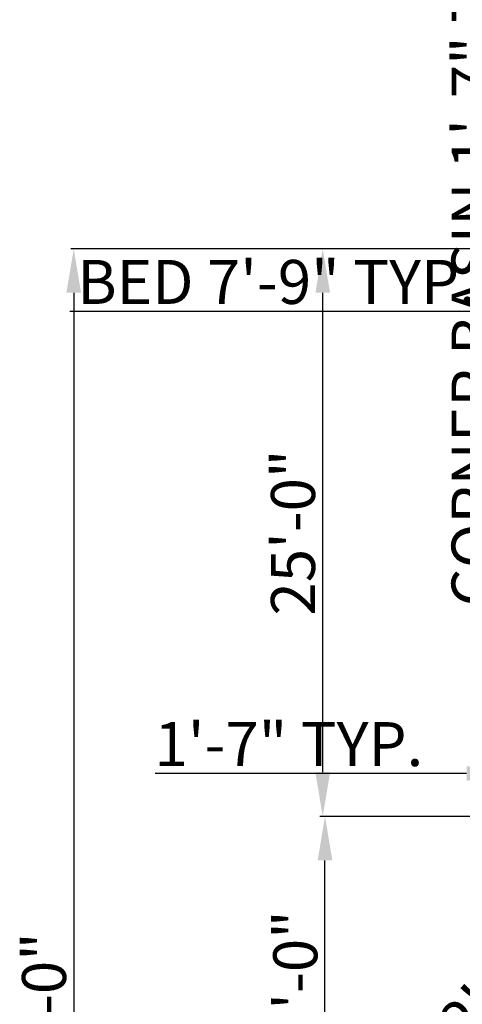
# Model space of a CAD drawing. Units: inches. Extents: x 2043 to 3177, y 1429 to 2563.
# Tile 9 of 14: x 2043 to 2224, y 1952 to 2355. Entities that reach past the tile are written whole.
import ezdxf

# ---------------------------------------------------------------- set-up
doc = ezdxf.new("R2010")
doc.units = ezdxf.units.IN
doc.layers.add('A-ANNO-DIMS', color=2, linetype='Continuous', lineweight=13)
doc.styles.get("Standard").update_dxf_attribs({"font": 'arial.ttf'})
doc.dimstyles.new('ISO-25', dxfattribs={"dimtxt": 18, "dimasz": 18, "dimexe": 1.25, "dimexo": 0.625, "dimtad": 1, "dimlunit": 3, "dimtxsty": 'Standard', "dimcen": 2.5, "dimadec": 0, "dimazin": 0, "dimtfac": 1, "dimtmove": 0, "dimatfit": 3, "dimfxl": 1, "dimarcsym": 0})

# ---------------------------------------------------------------- blocks, each defined once
blk = doc.blocks.new('*D26')
at = {"layer": 'A-ANNO-DIMS', "color": 0, "lineweight": -2, "transparency": 16777216}
for p, q in [((2233.12, 2029.27), (2166.79, 2029.27)), ((2168.04, 1902.52), (2168.04, 2011.27)), ((2233.12, 1884.52), (2166.79, 1884.52))]:
    blk.add_line(p, q, dxfattribs=at)
at = {"layer": 'A-ANNO-DIMS', "color": 0, "transparency": 16777216}
for points in [[(2165.04, 2011.27), (2171.04, 2011.27), (2168.04, 2029.27)], [(2165.04, 1902.52), (2171.04, 1902.52), (2168.04, 1884.52)]]:
    blk.add_solid(points, dxfattribs=at)
at = {"layer": 'Defpoints', "color": 0, "transparency": 16777216}
for p in [(2168.04, 2029.27), (2233.74, 2029.27), (2233.74, 1884.52)]:
    blk.add_point(p, dxfattribs=at)
at = {"layer": 'A-ANNO-DIMS', "color": 0, "transparency": 16777216, "insert": (2158.23, 1956.89), "char_height": 18, "attachment_point": 5, "rotation": 90}
blk.add_mtext('19\'-0"', dxfattribs=at)
blk = doc.blocks.new('*D27')
at = {"layer": 'A-ANNO-DIMS', "color": 0, "lineweight": -2, "transparency": 16777216}
for p, q in [((2233.12, 2261.39), (2165.87, 2261.39)), ((2167.12, 2047.27), (2167.12, 2243.39)), ((2233.12, 2029.27), (2165.87, 2029.27))]:
    blk.add_line(p, q, dxfattribs=at)
at = {"layer": 'A-ANNO-DIMS', "color": 0, "transparency": 16777216}
for points in [[(2164.12, 2243.39), (2170.12, 2243.39), (2167.12, 2261.39)], [(2164.12, 2047.27), (2170.12, 2047.27), (2167.12, 2029.27)]]:
    blk.add_solid(points, dxfattribs=at)
at = {"layer": 'Defpoints', "color": 0, "transparency": 16777216}
for p in [(2167.12, 2261.39), (2233.74, 2261.39), (2233.74, 2029.27)]:
    blk.add_point(p, dxfattribs=at)
at = {"layer": 'A-ANNO-DIMS', "color": 0, "transparency": 16777216, "insert": (2157.3, 2145.33), "char_height": 18, "attachment_point": 5, "rotation": 90}
blk.add_mtext('25\'-0"', dxfattribs=at)
blk = doc.blocks.new('*D28')
at = {"layer": 'A-ANNO-DIMS', "color": 0, "lineweight": -2, "transparency": 16777216}
for p, q in [((2233.12, 2261.39), (2064.1, 2261.39)), ((2065.35, 2243.39), (2065.35, 1652.39)), ((2233.12, 1634.39), (2064.1, 1634.39))]:
    blk.add_line(p, q, dxfattribs=at)
at = {"layer": 'A-ANNO-DIMS', "color": 0, "transparency": 16777216}
for points in [[(2062.35, 2243.39), (2068.35, 2243.39), (2065.35, 2261.39)], [(2062.35, 1652.39), (2068.35, 1652.39), (2065.35, 1634.39)]]:
    blk.add_solid(points, dxfattribs=at)
at = {"layer": 'Defpoints', "color": 0, "transparency": 16777216}
for p in [(2233.74, 2261.39), (2065.35, 1634.39), (2233.74, 1634.39)]:
    blk.add_point(p, dxfattribs=at)
at = {"layer": 'A-ANNO-DIMS', "color": 0, "transparency": 16777216, "insert": (2055.54, 1947.89), "char_height": 18, "attachment_point": 5, "rotation": 90}
blk.add_mtext('75\'-0"', dxfattribs=at)
blk = doc.blocks.new('*D53')
at = {"layer": 'A-ANNO-DIMS', "color": 0, "lineweight": -2, "transparency": 16777216}
for p, q in [((2250.66, 2235.7), (2063.8, 2235.7)), ((2250.66, 2222.4), (2250.66, 2236.95)), ((2325.44, 2235.7), (2268.66, 2235.7)), ((2343.44, 2222.4), (2343.44, 2236.95))]:
    blk.add_line(p, q, dxfattribs=at)
at = {"layer": 'A-ANNO-DIMS', "color": 0, "transparency": 16777216}
for points in [[(2268.66, 2238.7), (2268.66, 2232.7), (2250.66, 2235.7)], [(2325.44, 2238.7), (2325.44, 2232.7), (2343.44, 2235.7)]]:
    blk.add_solid(points, dxfattribs=at)
at = {"layer": 'Defpoints', "color": 0, "transparency": 16777216}
for p in [(2250.66, 2235.7), (2250.66, 2221.78), (2343.44, 2221.78)]:
    blk.add_point(p, dxfattribs=at)
at = {"layer": 'A-ANNO-DIMS', "color": 0, "transparency": 16777216, "insert": (2148.23, 2245.51), "char_height": 18, "attachment_point": 5}
blk.add_mtext('BED 7\'-9" TYP.', dxfattribs=at)
blk = doc.blocks.new('*D59')
at = {"layer": 'A-ANNO-DIMS', "color": 0, "lineweight": -2, "transparency": 16777216}
for p, q in [((2241.04, 2086.9), (2241.04, 2414.07)), ((2243.29, 2068.9), (2239.79, 2068.9)), ((2241.04, 2049.7), (2241.04, 2068.9)), ((2243.29, 2049.7), (2239.79, 2049.7)), ((2241.04, 2031.7), (2241.04, 2013.7))]:
    blk.add_line(p, q, dxfattribs=at)
at = {"layer": 'A-ANNO-DIMS', "color": 0, "transparency": 16777216}
for points in [[(2238.04, 2086.9), (2244.04, 2086.9), (2241.04, 2068.9)], [(2238.04, 2031.7), (2244.04, 2031.7), (2241.04, 2049.7)]]:
    blk.add_solid(points, dxfattribs=at)
at = {"layer": 'Defpoints', "color": 0, "transparency": 16777216}
for p in [(2241.04, 2068.9), (2243.92, 2068.9), (2243.92, 2049.7)]:
    blk.add_point(p, dxfattribs=at)
at = {"layer": 'A-ANNO-DIMS', "color": 0, "transparency": 16777216, "insert": (2231.1, 2259.48), "char_height": 18, "attachment_point": 5, "rotation": 90}
blk.add_mtext('CORNER BASIN 1\'-7" TYP.', dxfattribs=at)
blk = doc.blocks.new('*D60')
at = {"layer": 'A-ANNO-DIMS', "color": 0, "lineweight": -2, "transparency": 16777216}
for p, q in [((2225.92, 2046.82), (2098.64, 2046.82)), ((2243.92, 2049.08), (2243.92, 2045.57)), ((2263.12, 2046.82), (2243.92, 2046.82)), ((2263.12, 2049.08), (2263.12, 2045.57)), ((2281.12, 2046.82), (2299.12, 2046.82))]:
    blk.add_line(p, q, dxfattribs=at)
at = {"layer": 'A-ANNO-DIMS', "color": 0, "transparency": 16777216}
for points in [[(2225.92, 2049.82), (2225.92, 2043.82), (2243.92, 2046.82)], [(2281.12, 2049.82), (2281.12, 2043.82), (2263.12, 2046.82)]]:
    blk.add_solid(points, dxfattribs=at)
at = {"layer": 'Defpoints', "color": 0, "transparency": 16777216}
for p in [(2243.92, 2049.7), (2243.92, 2046.82), (2263.12, 2049.7)]:
    blk.add_point(p, dxfattribs=at)
at = {"layer": 'A-ANNO-DIMS', "color": 0, "transparency": 16777216, "insert": (2153.28, 2056.49), "char_height": 18, "attachment_point": 5}
blk.add_mtext('1\'-7" TYP.', dxfattribs=at)
blk = doc.blocks.new('*D92')
at = {"layer": 'A-ANNO-DIMS', "color": 0, "lineweight": -2, "transparency": 16777216}
for p, q in [((2351.56, 2062.42), (2327.82, 2037.29)), ((2219.16, 1922.24), (2315.46, 2024.21))]:
    blk.add_line(p, q, dxfattribs=at)
at = {"layer": 'A-ANNO-DIMS', "color": 0, "transparency": 16777216}
blk.add_solid([(2313.28, 2026.27), (2317.64, 2022.15), (2327.82, 2037.29)], dxfattribs=at)
at = {"layer": 'Defpoints', "color": 0, "transparency": 16777216}
for p in [(2351.56, 2062.42), (2327.82, 2037.29)]:
    blk.add_point(p, dxfattribs=at)
at = {"layer": 'A-ANNO-DIMS', "color": 0, "transparency": 16777216, "insert": (2253.91, 1973.5), "char_height": 18, "attachment_point": 5, "rotation": 46.6358}
blk.add_mtext('R2\'-10 1/2"', dxfattribs=at)

msp = doc.modelspace()

# ---------------------------------------------------------------- dimensions: what is measured, and where the dimension line sits
at = {"layer": 'A-ANNO-DIMS'}
for base, p1, p2, angle, text, override, picture, middle in [((2241.039, 2068.902), (2243.919, 2049.702), (2243.919, 2068.902), 90, 'CORNER BASIN <> TYP.', {"dimdec": 1, "dimlfac": 1, "dimrnd": 0, "dimzin": 1, "dimdsep": 46, "dimlunit": 4, "dimfrac": 2}, '*D59', (2231.101, 2259.485)), ((2250.662, 2235.697), (2343.44, 2221.78), (2250.662, 2221.78), 180, 'BED <> TYP.', {"dimdec": 1, "dimlfac": 1, "dimrnd": 0, "dimzin": 1, "dimdsep": 46, "dimlunit": 4, "dimfrac": 2}, '*D53', (2148.232, 2245.512)), ((2065.352, 1634.393), (2233.745, 2261.393), (2233.745, 1634.393), 90, '75\'-0"', {"dimclrd": 0, "dimclre": 0, "dimclrt": 0}, '*D28', (2055.537, 1947.893)), ((2167.117, 2261.393), (2233.745, 2029.268), (2233.745, 2261.393), 90, '25\'-0"', {"dimclrd": 0, "dimclre": 0, "dimclrt": 0}, '*D27', (2157.302, 2145.331)), ((2243.919, 2046.822), (2263.119, 2049.702), (2243.919, 2049.702), 180, '<> TYP.', {"dimdec": 1, "dimlfac": 1, "dimrnd": 0, "dimzin": 1, "dimdsep": 46, "dimlunit": 4, "dimfrac": 2}, '*D60', (2153.282, 2056.49)), ((2168.041, 2029.268), (2233.745, 1884.518), (2233.745, 2029.268), 90, '19\'-0"', {"dimclrd": 0, "dimclre": 0, "dimclrt": 0}, '*D26', (2158.225, 1956.893))]:
    dim = msp.add_linear_dim(base=base, p1=p1, p2=p2, angle=angle, text=text, dimstyle='ISO-25', override=override, dxfattribs=at)
    dim.commit()
    dim.dimension.update_dxf_attribs({"geometry": picture, "text_midpoint": middle})
dim = msp.add_radius_dim(center=(2351.556, 2062.422), mpoint=(2327.822, 2037.293), dimstyle='ISO-25', override={"dimdec": 1, "dimlfac": 1, "dimrnd": 0, "dimzin": 1, "dimdsep": 46, "dimlunit": 4, "dimfrac": 2}, dxfattribs=at)
dim.commit()
dim.dimension.update_dxf_attribs({"geometry": '*D92', "text_midpoint": (2253.911, 1973.501)})

doc.saveas('drawing.dxf')
